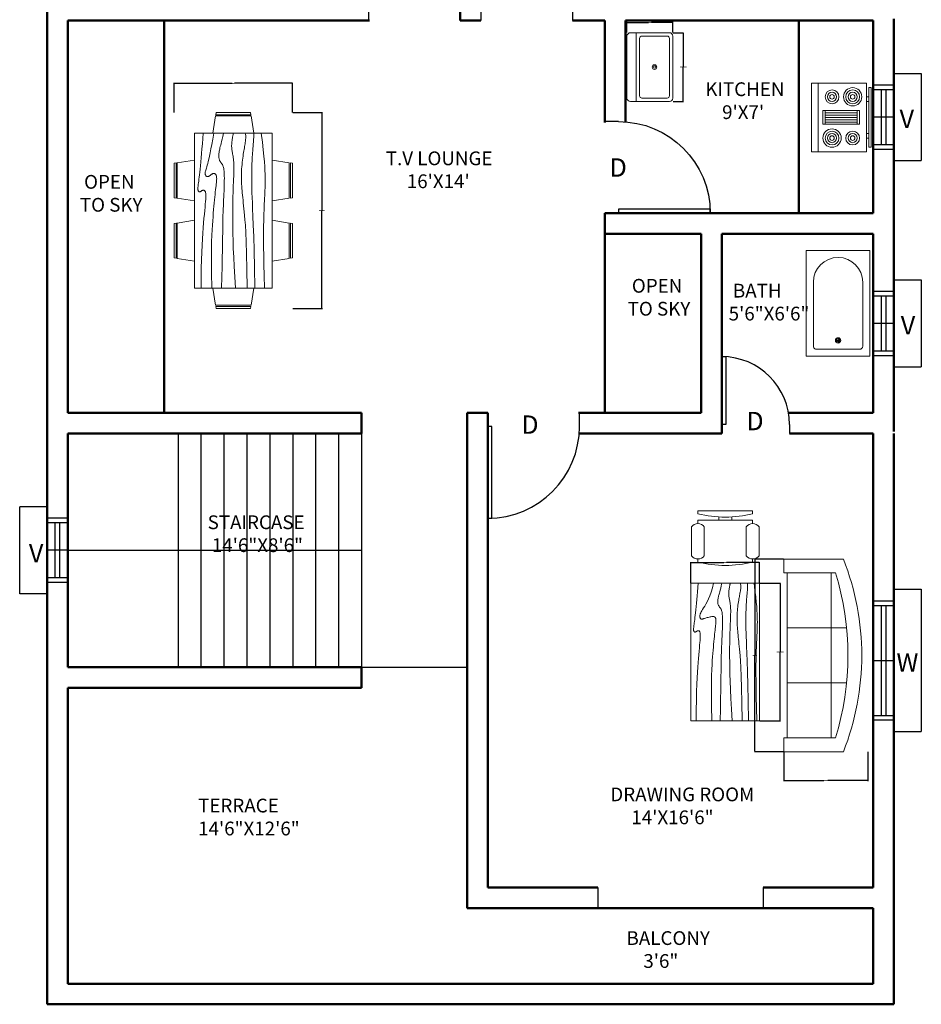
# Model space of a CAD drawing. Units: inches. Extents: x -8 to 1354, y -679 to 94.
# Tile 5 of 6: x 961 to 1354, y -679 to -249. Entities that reach past the tile are written whole.
import ezdxf

# ---------------------------------------------------------------- set-up
doc = ezdxf.new("R2010")
doc.units = ezdxf.units.IN
doc.header["$MEASUREMENT"] = 0
for name, color, linetype, lineweight in [('A-ANNO-DIMS', 2, 'Continuous', 18), ('A-ANNO-TEXT', 7, 'Continuous', 25), ('A-AREA-IDEN', 7, 'Continuous', 25), ('A-DOOR', 3, 'Continuous', 25), ('A-FLOR-FIXT', 8, 'Continuous', 18), ('A-FLOR-STRS', 2, 'Continuous', 25), ('A-FURN', 8, 'Continuous', 18), ('A-GLAZ', 4, 'Continuous', 25), ('A-WALL', 1, 'Continuous', 50)]:
    doc.layers.add(name, color=color, linetype=linetype, lineweight=lineweight)
doc.styles.get("Standard").update_dxf_attribs({"font": 'arial.ttf'})
doc.dimstyles.get("Standard").update_dxf_attribs({"dimtxt": 0.18, "dimasz": 0.18, "dimexe": 0.18, "dimexo": 0.0625, "dimgap": 0.09, "dimtad": 0, "dimtih": 1, "dimtoh": 1, "dimdec": 1, "dimzin": 0, "dimdsep": 46, "dimlunit": 4, "dimtxsty": 'Standard', "dimcen": 0.09, "dimclrd": 2, "dimclre": 3, "dimclrt": 6, "dimadec": 0, "dimazin": 0, "dimtfac": 1, "dimtdec": 1, "dimtofl": 0, "dimtmove": 0, "dimatfit": 3, "dimfxl": 1, "dimtfill": 2, "dimtfillclr": 4, "dimtolj": 1, "dimtzin": 0, "dimarcsym": 0})

# ---------------------------------------------------------------- blocks, each defined once
blk = doc.blocks.new('*U2')
for p, q in [((0, 0), (0, 6)), ((40, 0), (40, 6))]:
    blk.add_line(p, q)
blk.add_lwpolyline([(0, 0), (0, -40), (1.75, -40), (1.75, 0)], close=True)
blk.add_arc((0, 0), 40, 270, 0)
blk = doc.blocks.new('*U4')
for p, q in [((0, 0), (0, -100)), ((750, 0), (750, -100))]:
    blk.add_line(p, q)
blk.add_lwpolyline([(0, 0), (0, 750), (43.75, 750), (43.75, 0)], close=True)
blk.add_arc((0, 0), 750, 0, 90)
blk = doc.blocks.new('*U30')
for p, q in [((0, 0), (0, -6)), ((40, 0), (40, -6))]:
    blk.add_line(p, q)
blk.add_lwpolyline([(0, 0), (0, 40), (1.75, 40), (1.75, 0)], close=True)
blk.add_arc((0, 0), 40, 0, 90)
blk = doc.blocks.new('Sofa - Roundback 7 ft.')
for p, q in [((-12.00002, -32.4421), (-12.00003, -6.5971)), ((11.99997, -32.4421), (11.99998, -6.5971)), ((-36.000027, -34), (-36.000027, -11.4696)), ((35.99998, -34), (35.99998, -11.4696)), ((-35.999844, -13.3819), (35.9998, -13.3819)), ((-36.000027, -32.4421), (35.99998, -32.4421))]:
    blk.add_line(p, q)
for points in [[(-36.000027, -34), (-42.000027, -34), (-42.000027, -8)], [(41.99998, -8), (41.99998, -34), (35.99998, -34)]]:
    blk.add_lwpolyline(points)
for centre, radius, start, end in [((0, -114.25), 114.25, 68.43141, 111.5686), ((-0.00001, -127.1968), 121.1968, 72.72033, 107.2797)]:
    blk.add_arc(centre, radius, start, end)
blk = doc.blocks.new('Table - Rectangular Woodgrain 60 x 30 in.')
for p, q in [((0, 0), (0, -30)), ((60, 0), (0, 0)), ((60, -30), (60, 0)), ((0, -30), (60, -30))]:
    blk.add_line(p, q)
for points in [[(0, -2.4), (4.8155, -2.418), (9.0302, -2.4688), (12.709, -2.5477), (15.9167, -2.65), (18.7181, -2.7711), (21.1781, -2.9063), (23.3616, -3.0508), (25.3333, -3.2), (27.1477, -3.3495), (28.8172, -3.4958), (30.3437, -3.636), (31.7291, -3.7667), (32.9756, -3.8849), (34.0849, -3.9875), (35.059, -4.0714), (35.9, -4.1334), (36.6114, -4.1711), (37.2041, -4.1854), (37.6906, -4.1779), (38.0833, -4.15), (38.3948, -4.1034), (38.6375, -4.0396), (38.8239, -3.9602), (38.9666, -3.8667), (39.0764, -3.7608), (39.1573, -3.6448), (39.2116, -3.521), (39.2416, -3.3917), (39.2498, -3.2593), (39.2385, -3.1261), (39.21, -2.9944), (39.1666, -2.8667), (39.111, -2.7447), (39.0468, -2.6281), (38.978, -2.5163), (38.9083, -2.4083), (38.8418, -2.3035), (38.7823, -2.201), (38.7337, -2.1001), (38.7, -2), (38.6844, -1.9003), (38.6875, -1.8021), (38.7094, -1.707), (38.75, -1.6167), (38.8094, -1.5326), (38.8875, -1.4563), (38.9844, -1.3893), (39.1, -1.3333), (39.2351, -1.2896), (39.3937, -1.2583), (39.5804, -1.2396), (39.8, -1.2333), (40.057, -1.2396), (40.3562, -1.2583), (40.7023, -1.2896), (41.1, -1.3333), (41.5547, -1.3895), (42.0755, -1.4573), (42.6721, -1.5361), (43.3542, -1.625), (44.1316, -1.7233), (45.014, -1.8302), (46.0114, -1.9449), (47.1333, -2.0667), (48.3862, -2.1947), (49.7625, -2.3281), (51.2513, -2.4663), (52.8416, -2.6083), (54.5226, -2.7535), (56.2833, -2.9011), (58.1127, -3.0501), (60, -3.2)], [(0, -9.2), (6.5759, -9.0858), (11.9385, -9.0365), (16.2527, -9.0418), (19.6833, -9.0917), (22.3952, -9.1759), (24.5531, -9.2844), (26.322, -9.4069), (27.8666, -9.5333), (29.3241, -9.6553), (30.7203, -9.7719), (32.0532, -9.8837), (33.3208, -9.9917), (34.5213, -10.0965), (35.6526, -10.199), (36.7128, -10.2999), (37.7, -10.4), (38.6129, -10.4996), (39.4531, -10.5969), (40.223, -10.6895), (40.925, -10.775), (41.5613, -10.8512), (42.1344, -10.9156), (42.6465, -10.966), (43.1, -11), (43.4976, -11.0158), (43.8437, -11.0136), (44.143, -10.9942), (44.4, -10.9583), (44.6195, -10.9069), (44.8062, -10.8406), (44.9648, -10.7603), (45.1, -10.6667), (45.2155, -10.5598), (45.3114, -10.4365), (45.3871, -10.2929), (45.4416, -10.125), (45.4743, -9.929), (45.4844, -9.7011), (45.4709, -9.4371), (45.4333, -9.1333), (45.3716, -8.7883), (45.2896, -8.4104), (45.1919, -8.0107), (45.0833, -7.6), (44.9685, -7.1893), (44.8521, -6.7896), (44.7388, -6.4117), (44.6333, -6.0667), (44.54, -5.7628), (44.4614, -5.4979), (44.4001, -5.2675), (44.3583, -5.0667), (44.3384, -4.8909), (44.3427, -4.7354), (44.3736, -4.5956), (44.4333, -4.4667), (44.5236, -4.3453), (44.6427, -4.2333), (44.7884, -4.1339), (44.9583, -4.05), (45.1501, -3.9849), (45.3614, -3.9417), (45.59, -3.9234), (45.8333, -3.9333), (46.0915, -3.9749), (46.3734, -4.0531), (46.6906, -4.1736), (47.0542, -4.3417), (47.4756, -4.5629), (47.9661, -4.8427), (48.5372, -5.1866), (49.2, -5.6), (49.9676, -6.0844), (50.8594, -6.625), (51.8965, -7.2031), (53.1, -7.8), (54.491, -8.3969), (56.0906, -8.975), (57.9199, -9.5156), (60, -10)], [(0, -12.8), (5.1847, -12.9322), (9.6213, -13.0323), (13.3963, -13.1059), (16.5958, -13.1583), (19.3063, -13.1952), (21.614, -13.2219), (23.6054, -13.2439), (25.3666, -13.2667), (26.9728, -13.2947), (28.4531, -13.3281), (29.8256, -13.3663), (31.1083, -13.4083), (32.3191, -13.4535), (33.476, -13.501), (34.597, -13.5501), (35.7, -13.6), (36.7984, -13.6497), (37.8875, -13.6979), (38.9578, -13.743), (40, -13.7833), (41.0047, -13.8174), (41.9625, -13.8438), (42.864, -13.8607), (43.7, -13.8667), (44.4631, -13.8604), (45.1552, -13.8417), (45.7801, -13.8104), (46.3416, -13.7667), (46.8439, -13.7104), (47.2906, -13.6417), (47.6858, -13.5604), (48.0333, -13.4667), (48.3375, -13.3608), (48.6042, -13.2448), (48.8396, -13.121), (49.05, -12.9917), (49.2417, -12.8593), (49.4208, -12.7261), (49.5937, -12.5944), (49.7667, -12.4667), (49.9452, -12.3451), (50.1323, -12.2313), (50.3303, -12.1268), (50.5416, -12.0333), (50.7686, -11.9524), (51.0135, -11.8854), (51.2788, -11.8341), (51.5666, -11.8), (51.8785, -11.7843), (52.2116, -11.7865), (52.562, -11.8059), (52.926, -11.8417), (53.2998, -11.8931), (53.6795, -11.9594), (54.0614, -12.0397), (54.4416, -12.1333), (54.8223, -12.2401), (55.2293, -12.3625), (55.6942, -12.5037), (56.2489, -12.6667), (56.9251, -12.8547), (57.7545, -13.0708), (58.7689, -13.3182), (60, -13.6)], [(0, -18), (5.124, -17.7273), (9.6609, -17.5057), (13.6705, -17.3303), (17.2125, -17.1958), (20.3467, -17.0973), (23.1328, -17.0297), (25.6307, -16.9878), (27.9, -16.9667), (29.9928, -16.9617), (31.9302, -16.9703), (33.7254, -16.9907), (35.3917, -17.0208), (36.9423, -17.0588), (38.3906, -17.1026), (39.7499, -17.1503), (41.0333, -17.2), (42.2519, -17.2496), (43.4073, -17.2969), (44.4986, -17.3395), (45.525, -17.375), (46.4858, -17.4012), (47.3802, -17.4156), (48.2074, -17.416), (48.9667, -17.4), (49.6583, -17.3662), (50.2872, -17.3167), (50.8595, -17.2547), (51.3812, -17.1833), (51.8584, -17.1057), (52.2971, -17.025), (52.7034, -16.9443), (53.0833, -16.8667), (53.443, -16.7951), (53.789, -16.7313), (54.128, -16.6768), (54.4666, -16.6334), (54.8115, -16.6024), (55.1693, -16.5854), (55.5465, -16.5841), (55.95, -16.6), (56.3828, -16.6337), (56.8346, -16.6823), (57.2915, -16.7418), (57.7396, -16.8084), (58.165, -16.878), (58.5539, -16.9469), (58.8924, -17.0111), (59.1666, -17.0667), (59.3679, -17.1107), (59.5078, -17.1438), (59.6032, -17.1675), (59.6708, -17.1833), (59.7275, -17.193), (59.7901, -17.1979), (59.8753, -17.1998), (60, -17.2)], [(0, -22.4), (8.0098, -22.2501), (14.4094, -22.1011), (19.4168, -21.9535), (23.25, -21.8083), (26.1269, -21.6663), (28.2656, -21.5281), (29.884, -21.3947), (31.2, -21.2667), (32.3967, -21.1448), (33.5172, -21.0292), (34.5697, -20.9198), (35.5625, -20.8167), (36.5037, -20.7198), (37.4015, -20.6292), (38.2642, -20.5448), (39.1, -20.4667), (39.9164, -20.3951), (40.7187, -20.3313), (41.5117, -20.2768), (42.3, -20.2333), (43.0883, -20.2024), (43.8812, -20.1854), (44.6836, -20.1841), (45.5, -20.2), (46.3328, -20.234), (47.1747, -20.2844), (48.0163, -20.3488), (48.8479, -20.425), (49.66, -20.5106), (50.4429, -20.6031), (51.1872, -20.7004), (51.8833, -20.8), (52.5246, -20.8999), (53.1166, -20.9995), (53.6681, -21.0983), (54.1875, -21.1958), (54.6834, -21.2919), (55.1646, -21.3859), (55.6394, -21.4777), (56.1167, -21.5667), (56.6028, -21.6515), (57.0961, -21.7266), (57.5929, -21.7852), (58.0896, -21.8208), (58.5823, -21.8268), (59.0674, -21.7964), (59.5412, -21.723), (60, -21.6)], [(0, -25.2), (8.6355, -25.0504), (15.7026, -24.9031), (21.4049, -24.7606), (25.9458, -24.625), (29.529, -24.4988), (32.3578, -24.3844), (34.6359, -24.284), (36.5667, -24.2), (38.3213, -24.1341), (39.9417, -24.0854), (41.437, -24.0523), (42.8167, -24.0333), (44.0901, -24.0268), (45.2667, -24.0313), (46.3557, -24.0451), (47.3667, -24.0667), (48.309, -24.0947), (49.1928, -24.1287), (50.0284, -24.168), (50.826, -24.2125), (51.5959, -24.2617), (52.3483, -24.3151), (53.0935, -24.3725), (53.8417, -24.4334), (54.6009, -24.497), (55.3699, -24.561), (56.1454, -24.6226), (56.9239, -24.6792), (57.7021, -24.7279), (58.4764, -24.7662), (59.2435, -24.7911), (60, -24.8)], [(0, -28.8), (5.6867, -28.6681), (10.45, -28.5698), (14.407, -28.5012), (17.675, -28.4584), (20.3711, -28.4374), (22.6125, -28.4344), (24.5164, -28.4455), (26.2, -28.4667), (27.762, -28.4947), (29.2276, -28.5281), (30.6033, -28.5663), (31.8958, -28.6084), (33.1118, -28.6535), (34.2578, -28.7011), (35.3405, -28.7501), (36.3666, -28.8), (37.3443, -28.8497), (38.288, -28.8974), (39.2137, -28.9412), (40.1375, -28.9792), (41.0753, -29.0093), (42.0432, -29.0297), (43.0572, -29.0384), (44.1333, -29.0333), (45.2936, -29.0114), (46.5843, -28.9641), (48.0579, -28.8816), (49.7666, -28.7542), (51.7629, -28.5721), (54.0989, -28.3255), (56.8272, -28.0048), (60, -27.6)]]:
    blk.add_lwpolyline(points)
blk = doc.blocks.new('Chair - Desk')
for p, q in [((-8.5, 0), (-8.5, -1)), ((-8.5, 0), (8.5, 0)), ((8.5, 0), (8.5, -1)), ((-8.5, -3), (-8.5, -4)), ((-8.5, -3), (8.5, -3)), ((-2, -3), (-2, -1.9355)), ((2, -1.9576), (2, -3)), ((8.5, -3), (8.5, -4)), ((-10.5, -5), (-10.5, -14)), ((-6.5, -14), (-6.5, -5)), ((6.5, -5), (6.5, -14)), ((10.5, -14), (10.5, -5)), ((-8.5, -15), (-8.5, -16)), ((8.5, -15), (8.5, -16))]:
    blk.add_line(p, q)
for centre, radius, start, end in [((0, 34.625), 36.625, 256.5803, 283.4197), ((-8.5, -6.5), 2.5, 36.8699, 143.1301), ((8.5, -6.5), 2.5, 36.8699, 143.1301), ((-8.5, -12.5), 2.5, 216.8699, 323.1301), ((8.5, -12.5), 2.5, 216.8699, 323.1301), ((0, 19.625), 36.625, 256.5803, 283.4197)]:
    blk.add_arc(centre, radius, start, end)
blk = doc.blocks.new('Bath Tub - 26 x 60 in.')
for p, q in [((8, -18), (10, -18)), ((9, -17), (9, -19))]:
    blk.add_line(p, q)
blk.add_lwpolyline([(0, -36), (0, 0), (60, 0), (60, -36)], close=True)
for points in [[(6, -4), (42, -4)], [(4, -30), (4, -6)], [(42, -32), (6, -32)]]:
    blk.add_lwpolyline(points)
for radius in [1.5, 1]:
    blk.add_circle((9, -18), radius)
for centre, radius, start, end in [((5.75, -5.75), 1.77, 81.8699, 188.1301), ((42, -18), 14, 270, 90), ((5.75, -30.25), 1.77, 171.8699, 278.1301)]:
    blk.add_arc(centre, radius, start, end)
blk = doc.blocks.new('Range-Oven - 30 in top')
for p, q in [((0, -3), (30, -3)), ((12, -6), (18, -6)), ((13, -20), (13, -6)), ((14, -6), (14, -20)), ((15, -20), (15, -6)), ((16, -6), (16, -20)), ((17, -20), (17, -6)), ((18, -20), (12, -20)), ((6, -24), (6, -25)), ((8, -25), (8, -24)), ((22, -25), (22, -24)), ((24, -24), (24, -25))]:
    blk.add_line(p, q)
for points in [[(0, -24), (0, 0), (30, 0), (30, -24)], [(12, -21), (12, -5), (18, -5), (18, -21)], [(2, -26), (2, -25), (28, -25), (28, -26)]]:
    blk.add_lwpolyline(points, close=True)
for centre, radius in [((6, -9), 4), ((6, -9), 3), ((6, -9), 2), ((6, -9), 1), ((24, -9), 3), ((24, -9), 2), ((24, -9), 1), ((6, -18), 3), ((6, -18), 2), ((6, -18), 1), ((24, -18), 4), ((24, -18), 3), ((24, -18), 2), ((24, -18), 1)]:
    blk.add_circle(centre, radius)
blk = doc.blocks.new('Sink-single - 30 in top')
blk.add_line((-15, -3.999996), (15, -3.999996))
for points in [[(-13.5, 0), (13.5, 0)], [(-15, -18.499996), (-15, -1.5)], [(15, -1.5), (15, -18.499996)], [(-13.5, -17.499996), (-13.5, -6.499996)], [(-12.5, -5.499996), (12.5, -5.499996)], [(13.5, -6.499996), (13.5, -17.499996)], [(13.5, -19.999996), (-13.5, -19.999996)], [(12.5, -18.499996), (-12.5, -18.499996)]]:
    blk.add_lwpolyline(points)
for radius in [1, 0.5]:
    blk.add_circle((0, -11.999996), radius)
for centre, radius, start, end in [((-13.5, -1.5), 1.5, 90, 180), ((13.5, -1.5), 1.5, 0, 90), ((-12.5, -6.499996), 1, 90, 180), ((12.5, -6.499996), 1, 0, 90), ((-13.5, -18.499996), 1.5, 180, 270), ((-12.5, -17.499996), 1, 180, 270), ((12.5, -17.499996), 1, 270, 0), ((13.5, -18.499996), 1.5, 270, 0)]:
    blk.add_arc(centre, radius, start, end)
blk = doc.blocks.new('Dining Set - 36 x 72 in.')
for p, q in [((-22, 27.5), (-22.1562, 26.50042)), ((-22, 27.5), (-6, 27.5)), ((-5.8437, 26.49966), (-6, 27.5)), ((6, 27.5), (5.8438, 26.50042)), ((6, 27.5), (22, 27.5)), ((22.1563, 26.49966), (22, 27.5)), ((-22.2343, 26.00059), (-23.4847, 17.99762)), ((-22.2304, 26), (-5.7608, 26)), ((-5.8416, 26.5), (-22.1534, 26.5)), ((-4.5152, 17.99762), (-5.7655, 25.99926)), ((5.7657, 26.00059), (4.5153, 17.99762)), ((5.7696, 26), (22.2392, 26)), ((22.1584, 26.5), (5.8466, 26.5)), ((23.4848, 17.99762), (22.2345, 25.99926)), ((36, 18), (-36, 18)), ((-36, 18), (-36, -18)), ((36, -18), (36, 18)), ((-44.0006, 8.23428), (-35.9976, 9.48474)), ((44.0006, 8.23428), (35.9976, 9.48474)), ((-45.5, 8), (-44.5004, 8.15617)), ((-45.5, 8), (-45.5, -8)), ((-44.5, -8.15843), (-44.5, 8.15338)), ((-44, 8.23041), (-44, -8.23915)), ((44, 8.23041), (44, -8.23915)), ((44.5, -8.15843), (44.5, 8.15338)), ((45.5, 8), (44.5005, 8.15617)), ((45.5, 8), (45.5, -8)), ((-44.4997, -8.15631), (-45.5, -8)), ((-35.9976, -9.48476), (-43.9993, -8.2345)), ((35.9976, -9.48476), (43.9993, -8.2345)), ((44.4997, -8.15631), (45.5, -8)), ((-36, -18), (36, -18)), ((-22.2343, -26.0006), (-23.4847, -17.99762)), ((-4.5152, -17.99762), (-5.7655, -25.99928)), ((5.7657, -26.0006), (4.5153, -17.99762)), ((23.4848, -17.99762), (22.2345, -25.99928)), ((-22.2304, -26), (-5.7608, -26)), ((-22, -27.5), (-22.1562, -26.50044)), ((-5.8416, -26.5), (-22.1534, -26.5)), ((-5.8437, -26.49967), (-6, -27.5)), ((5.7696, -26), (22.2392, -26)), ((6, -27.5), (5.8438, -26.50044)), ((22.1584, -26.5), (5.8466, -26.5)), ((22.1563, -26.49967), (22, -27.5)), ((-22, -27.5), (-6, -27.5)), ((6, -27.5), (22, -27.5))]:
    blk.add_line(p, q)
for points in [[(-36, 15), (-31.1772, 14.97754), (-26.8079, 14.91406), (-22.8538, 14.81543), (-19.276, 14.6875), (-16.0362, 14.53613), (-13.0957, 14.36718), (-10.4159, 14.18652), (-7.9583, 14), (-5.6904, 13.81315), (-3.6035, 13.63021), (-1.6954, 13.45508), (0.0365, 13.29166), (1.5945, 13.14388), (2.9811, 13.01562), (4.1988, 12.9108), (5.25, 12.83333), (6.1393, 12.78613), (6.8802, 12.76823), (7.4883, 12.77767), (7.9792, 12.8125), (8.3685, 12.87077), (8.6719, 12.95052), (8.9049, 13.0498), (9.0833, 13.16666), (9.2205, 13.29899), (9.3216, 13.44401), (9.3895, 13.59879), (9.4271, 13.76041), (9.4373, 13.92594), (9.4232, 14.09245), (9.3875, 14.257), (9.3333, 14.41666), (9.2638, 14.56917), (9.1836, 14.71484), (9.0975, 14.85465), (9.0104, 14.98958), (8.9272, 15.1206), (8.8529, 15.2487), (8.7922, 15.37483), (8.75, 15.5), (8.7305, 15.62467), (8.7344, 15.74739), (8.7617, 15.86621), (8.8125, 15.97916), (8.8867, 16.08431), (8.9844, 16.17968), (9.1055, 16.26334), (9.25, 16.33333), (9.4189, 16.38802), (9.6172, 16.42708), (9.8506, 16.45052), (10.125, 16.45833), (10.4463, 16.45052), (10.8203, 16.42708), (11.2529, 16.38802), (11.75, 16.33333), (12.3184, 16.26318), (12.9694, 16.17838), (13.7151, 16.07991), (14.5677, 15.96875), (15.5395, 15.84586), (16.6426, 15.71224), (17.8893, 15.56884), (19.2917, 15.41666), (20.859, 15.25667), (22.5879, 15.08984), (24.4721, 14.91715), (26.5052, 14.73958), (28.6809, 14.5581), (30.9929, 14.3737), (33.4347, 14.18733), (36, 14)], [(-36, 10), (-28.9766, 10.14274), (-23.1725, 10.20442), (-18.4241, 10.19775), (-14.5677, 10.13541), (-11.4399, 10.03011), (-8.877, 9.89453), (-6.7154, 9.74137), (-4.7917, 9.58333), (-2.9698, 9.43082), (-1.2246, 9.28515), (0.4415, 9.14534), (2.026, 9.01041), (3.5266, 8.87939), (4.9408, 8.7513), (6.266, 8.62516), (7.5, 8.5), (8.6411, 8.37549), (9.6914, 8.2539), (10.6538, 8.13818), (11.5312, 8.03125), (12.3267, 7.93603), (13.043, 7.85547), (13.6831, 7.79248), (14.25, 7.75), (14.7471, 7.7303), (15.1797, 7.73307), (15.5537, 7.75732), (15.875, 7.80208), (16.1494, 7.86637), (16.3828, 7.94922), (16.5811, 8.04964), (16.75, 8.16666), (16.8944, 8.29915), (17.0143, 8.44531), (17.1089, 8.60319), (17.1771, 8.77083), (17.218, 8.94629), (17.2305, 9.1276), (17.2137, 9.31282), (17.1667, 9.5), (17.0895, 9.6875), (16.987, 9.875), (16.8649, 10.0625), (16.7292, 10.25), (16.5856, 10.4375), (16.4401, 10.625), (16.2985, 10.8125), (16.1667, 11), (16.05, 11.18733), (15.9518, 11.3737), (15.8752, 11.5581), (15.8229, 11.73958), (15.798, 11.91715), (15.8034, 12.08984), (15.842, 12.25667), (15.9167, 12.41666), (16.0295, 12.56836), (16.1784, 12.70833), (16.3605, 12.83268), (16.5729, 12.9375), (16.8127, 13.01888), (17.0768, 13.07291), (17.3625, 13.0957), (17.6667, 13.08333), (17.9894, 13.03312), (18.3418, 12.94726), (18.7382, 12.82918), (19.1927, 12.68229), (19.7195, 12.51001), (20.3327, 12.31575), (21.0465, 12.10294), (21.875, 11.875), (22.8357, 11.63354), (23.959, 11.37304), (25.2786, 11.08618), (26.8282, 10.76562), (28.6414, 10.40405), (30.752, 9.99414), (33.1936, 9.52856), (36, 9)], [(-36, 5.5), (-30.7157, 5.3348), (-26.069, 5.20963), (-21.9946, 5.11767), (-18.4271, 5.05208), (-15.3009, 5.00602), (-12.5508, 4.97265), (-10.1112, 4.94515), (-7.9167, 4.91666), (-5.909, 4.88167), (-4.0586, 4.83984), (-2.3429, 4.79215), (-0.7396, 4.73958), (0.7739, 4.6831), (2.22, 4.6237), (3.6213, 4.56233), (5, 4.5), (6.373, 4.43782), (7.7344, 4.3776), (9.0723, 4.32129), (10.375, 4.27083), (11.6309, 4.22819), (12.8281, 4.19531), (13.9551, 4.17415), (15, 4.16666), (15.954, 4.17448), (16.819, 4.19791), (17.6001, 4.23698), (18.3021, 4.29166), (18.9299, 4.36198), (19.4883, 4.44791), (19.9823, 4.54948), (20.4167, 4.66666), (20.7969, 4.79899), (21.1302, 4.94401), (21.4245, 5.09879), (21.6875, 5.26041), (21.9271, 5.42594), (22.1511, 5.59245), (22.3672, 5.757), (22.5834, 5.91666), (22.8065, 6.06868), (23.0404, 6.21093), (23.2879, 6.34147), (23.5521, 6.45833), (23.8358, 6.55957), (24.142, 6.64323), (24.4735, 6.70735), (24.8334, 6.75), (25.2235, 6.76969), (25.642, 6.76692), (26.0858, 6.74267), (26.5521, 6.69791), (27.0379, 6.63362), (27.5404, 6.55078), (28.0565, 6.45036), (28.5834, 6.33333), (29.1242, 6.19987), (29.7071, 6.04687), (30.3661, 5.87044), (31.1354, 5.66666), (32.0493, 5.43164), (33.142, 5.16146), (34.4475, 4.85221), (36, 4.5)], [(-36, -1), (-30.7915, -0.6591), (-26.0195, -0.38216), (-21.6519, -0.16284), (-17.6563, 0.00521), (-14.0005, 0.12833), (-10.6523, 0.21289), (-7.5796, 0.26522), (-4.75, 0.29166), (-2.134, 0.29793), (0.2878, 0.28711), (2.5317, 0.26163), (4.6146, 0.22396), (6.5529, 0.17651), (8.3633, 0.12174), (10.0623, 0.06209), (11.6667, 0), (13.1899, -0.06201), (14.6341, -0.1211), (15.9982, -0.17432), (17.2813, -0.21875), (18.4823, -0.25147), (19.6003, -0.26953), (20.6343, -0.27002), (21.5834, -0.25), (22.4481, -0.20768), (23.2357, -0.14584), (23.9549, -0.06836), (24.6146, 0.02083), (25.2235, 0.11784), (25.7904, 0.21875), (26.3241, 0.31966), (26.8334, 0.41666), (27.3265, 0.50618), (27.8099, 0.58593), (28.2894, 0.65397), (28.7709, 0.70833), (29.2601, 0.74707), (29.763, 0.76823), (30.2855, 0.76985), (30.8334, 0.75), (31.4088, 0.70784), (31.9994, 0.64713), (32.589, 0.57275), (33.1615, 0.48958), (33.7008, 0.4025), (34.1908, 0.3164), (34.6153, 0.23616), (34.9584, 0.16666), (35.2099, 0.11165), (35.3848, 0.07031), (35.504, 0.04069), (35.5886, 0.02083), (35.6594, 0.00879), (35.7377, 0.0026), (35.8442, 0.00032), (36, 0)], [(-36, -6.5), (-27.1843, -6.31267), (-20.084, -6.1263), (-14.469, -5.9419), (-10.1094, -5.76042), (-6.7752, -5.58285), (-4.2363, -5.41016), (-2.2629, -5.24333), (-0.625, -5.08334), (0.8708, -4.93099), (2.2715, -4.78646), (3.5872, -4.64974), (4.8281, -4.52084), (6.0046, -4.39974), (7.127, -4.28646), (8.2053, -4.18099), (9.25, -4.08334), (10.2705, -3.99382), (11.2734, -3.91407), (12.2647, -3.84603), (13.25, -3.79167), (14.2354, -3.75293), (15.2266, -3.73177), (16.2295, -3.73015), (17.25, -3.75), (18.2912, -3.79248), (19.3451, -3.85547), (20.4009, -3.93604), (21.4479, -4.03125), (22.4754, -4.13819), (23.4727, -4.25391), (24.4289, -4.37549), (25.3334, -4.5), (26.1785, -4.62492), (26.9694, -4.74935), (27.7145, -4.87281), (28.4219, -4.99479), (29.1, -5.11483), (29.7572, -5.23242), (30.4016, -5.34709), (31.0417, -5.45834), (31.6837, -5.56437), (32.3262, -5.65821), (32.9658, -5.73153), (33.599, -5.77604), (34.2224, -5.78345), (34.8327, -5.74545), (35.4264, -5.65373), (36, -5.5)], [(-36, -10), (-26.4022, -9.81299), (-18.4675, -9.62891), (-11.9839, -9.45069), (-6.7396, -9.28125), (-2.5226, -9.12354), (0.8789, -8.98047), (3.6769, -8.85498), (6.0833, -8.75), (8.2767, -8.66765), (10.3021, -8.60677), (12.1712, -8.56543), (13.8958, -8.54167), (15.4876, -8.53353), (16.9583, -8.53907), (18.3197, -8.55632), (19.5834, -8.58334), (20.7616, -8.61841), (21.8685, -8.66081), (22.9188, -8.71004), (23.9271, -8.76563), (24.9081, -8.82707), (25.8763, -8.89388), (26.8465, -8.96558), (27.8334, -9.04167), (28.8474, -9.12118), (29.8828, -9.20117), (30.93, -9.27824), (31.9792, -9.34896), (33.0205, -9.40991), (34.0443, -9.45768), (35.0407, -9.48885), (36, -9.5)], [(-36, -14.5), (-30.0881, -14.33513), (-25.0332, -14.21224), (-20.7312, -14.12647), (-17.0781, -14.07292), (-13.97, -14.04671), (-11.3027, -14.04297), (-8.9724, -14.05681), (-6.875, -14.08334), (-4.9224, -14.11833), (-3.0905, -14.16016), (-1.3709, -14.20785), (0.2448, -14.26042), (1.7647, -14.3169), (3.1973, -14.3763), (4.5507, -14.43767), (5.8333, -14.5), (7.0554, -14.5621), (8.235, -14.62175), (9.3922, -14.67652), (10.5469, -14.72396), (11.7192, -14.76164), (12.929, -14.78711), (14.1965, -14.79794), (15.5417, -14.79167), (16.9933, -14.76424), (18.6152, -14.70508), (20.4804, -14.60197), (22.6615, -14.44271), (25.2312, -14.21509), (28.2624, -13.9069), (31.8277, -13.50594), (36, -13)]]:
    blk.add_lwpolyline(points)
blk = doc.blocks.new('WIN-W')
at = {"ltscale": 2}
for p, q in [((12, 62), (0, 62)), ((0, 0), (0, 62)), ((12, 57), (12, 62)), ((12, 5), (12, 0)), ((12, 0), (0, 0))]:
    blk.add_line(p, q, dxfattribs=at)
for p, q in [((21, 57), (12, 57)), ((21, 5), (12, 5))]:
    blk.add_line(p, q)
blk = doc.blocks.new('VENT-V')
for p, q in [((0, 9), (0, 21)), ((0, 21), (38, 21)), ((38, 9), (38, 21)), ((5, 9), (0, 9)), ((5, 0), (5, 9)), ((33, 0), (33, 9)), ((33, 9), (38, 9))]:
    blk.add_line(p, q)
blk = doc.blocks.new('*D101')
at = {"layer": 'A-ANNO-DIMS', "color": 3, "lineweight": -2, "transparency": 16777216}
for p, q in [((1283.34, -494.98), (1292.45, -494.98)), ((1283.34, -554.98), (1292.45, -554.98))]:
    blk.add_line(p, q, dxfattribs=at)
at = {"layer": 'A-ANNO-DIMS', "color": 2, "lineweight": -2, "transparency": 16777216}
for p, q in [((1292.27, -495.16), (1292.27, -524.79)), ((1292.27, -554.8), (1292.27, -525.16))]:
    blk.add_line(p, q, dxfattribs=at)
at = {"layer": 'A-ANNO-DIMS', "color": 2, "transparency": 16777216}
for points in [[(1292.24, -495.16), (1292.3, -495.16), (1292.27, -494.98)], [(1292.24, -554.8), (1292.3, -554.8), (1292.27, -554.98)]]:
    blk.add_solid(points, dxfattribs=at)
at = {"layer": 'Defpoints', "color": 0, "transparency": 16777216}
for p in [(1283.27, -494.98), (1292.27, -494.98), (1283.27, -554.98)]:
    blk.add_point(p, dxfattribs=at)
at = {"layer": 'A-ANNO-DIMS', "color": 6, "transparency": 16777216, "insert": (1292.27, -524.98), "char_height": 0.18, "attachment_point": 5, "bg_fill": 1, "box_fill_scale": 1.25, "bg_fill_color": 4, "bg_fill_transparency": 0}
blk.add_mtext('\\A1;COFFEE TABLE 5\'-0" TYP.', dxfattribs=at)
blk = doc.blocks.new('*D102')
at = {"layer": 'A-ANNO-DIMS', "color": 3, "lineweight": -2, "transparency": 16777216}
for p, q in [((1253.27, -494.91), (1253.27, -485.8)), ((1283.27, -494.91), (1283.27, -485.8))]:
    blk.add_line(p, q, dxfattribs=at)
at = {"layer": 'A-ANNO-DIMS', "color": 2, "lineweight": -2, "transparency": 16777216}
for p, q in [((1253.45, -485.98), (1267.63, -485.98)), ((1283.09, -485.98), (1268.91, -485.98))]:
    blk.add_line(p, q, dxfattribs=at)
at = {"layer": 'A-ANNO-DIMS', "color": 2, "transparency": 16777216}
for points in [[(1253.45, -485.95), (1253.45, -486.01), (1253.27, -485.98)], [(1283.09, -485.95), (1283.09, -486.01), (1283.27, -485.98)]]:
    blk.add_solid(points, dxfattribs=at)
at = {"layer": 'Defpoints', "color": 0, "transparency": 16777216}
for p in [(1253.27, -485.98), (1253.27, -494.98), (1283.27, -494.98)]:
    blk.add_point(p, dxfattribs=at)
at = {"layer": 'A-ANNO-DIMS', "color": 6, "transparency": 16777216, "insert": (1268.27, -485.98), "char_height": 0.18, "attachment_point": 5, "bg_fill": 1, "box_fill_scale": 1.25, "bg_fill_color": 4, "bg_fill_transparency": 0}
blk.add_mtext('\\A1;2\'-6" TYP.', dxfattribs=at)
blk = doc.blocks.new('*D105')
at = {"layer": 'A-ANNO-DIMS', "color": 3, "lineweight": -2, "transparency": 16777216}
for p, q in [((1079.77, -289.78), (1092.7, -289.78)), ((1079.77, -375.2), (1092.7, -375.2))]:
    blk.add_line(p, q, dxfattribs=at)
at = {"layer": 'A-ANNO-DIMS', "color": 2, "lineweight": -2, "transparency": 16777216}
for p, q in [((1092.52, -289.96), (1092.52, -332.31)), ((1092.52, -375.02), (1092.52, -332.68))]:
    blk.add_line(p, q, dxfattribs=at)
at = {"layer": 'A-ANNO-DIMS', "color": 2, "transparency": 16777216}
for points in [[(1092.49, -289.96), (1092.55, -289.96), (1092.52, -289.78)], [(1092.49, -375.02), (1092.55, -375.02), (1092.52, -375.2)]]:
    blk.add_solid(points, dxfattribs=at)
at = {"layer": 'Defpoints', "color": 0, "transparency": 16777216}
for p in [(1079.7, -289.78), (1092.52, -289.78), (1079.7, -375.2)]:
    blk.add_point(p, dxfattribs=at)
at = {"layer": 'A-ANNO-DIMS', "color": 6, "transparency": 16777216, "insert": (1092.52, -332.49), "char_height": 0.18, "attachment_point": 5, "bg_fill": 1, "box_fill_scale": 1.25, "bg_fill_color": 4, "bg_fill_transparency": 0}
blk.add_mtext('\\A1;DINING SET 7\'-1 1/2"', dxfattribs=at)
blk = doc.blocks.new('*D106')
at = {"layer": 'A-ANNO-DIMS', "color": 3, "lineweight": -2, "transparency": 16777216}
for p, q in [((1028.08, -289.72), (1028.08, -276.79)), ((1079.7, -289.72), (1079.7, -276.79))]:
    blk.add_line(p, q, dxfattribs=at)
at = {"layer": 'A-ANNO-DIMS', "color": 2, "lineweight": -2, "transparency": 16777216}
for p, q in [((1028.26, -276.97), (1053.35, -276.97)), ((1079.52, -276.97), (1054.43, -276.97))]:
    blk.add_line(p, q, dxfattribs=at)
at = {"layer": 'A-ANNO-DIMS', "color": 2, "transparency": 16777216}
for points in [[(1028.26, -276.94), (1028.26, -277), (1028.08, -276.97)], [(1079.52, -276.94), (1079.52, -277), (1079.7, -276.97)]]:
    blk.add_solid(points, dxfattribs=at)
at = {"layer": 'Defpoints', "color": 0, "transparency": 16777216}
for p in [(1028.08, -276.97), (1028.08, -289.78), (1079.7, -289.78)]:
    blk.add_point(p, dxfattribs=at)
at = {"layer": 'A-ANNO-DIMS', "color": 6, "transparency": 16777216, "insert": (1053.89, -276.97), "char_height": 0.18, "attachment_point": 5, "bg_fill": 1, "box_fill_scale": 1.25, "bg_fill_color": 4, "bg_fill_transparency": 0}
blk.add_mtext('\\A1;4\'-3 1/2"', dxfattribs=at)
blk = doc.blocks.new('*D109')
at = {"layer": 'A-ANNO-DIMS', "color": 3, "lineweight": -2, "transparency": 16777216}
for p, q in [((1245.55, -254.9), (1250.17, -254.9)), ((1245.55, -284.9), (1250.17, -284.9))]:
    blk.add_line(p, q, dxfattribs=at)
at = {"layer": 'A-ANNO-DIMS', "color": 2, "lineweight": -2, "transparency": 16777216}
for p, q in [((1249.99, -255.08), (1249.99, -269.72)), ((1249.99, -284.72), (1249.99, -270.08))]:
    blk.add_line(p, q, dxfattribs=at)
at = {"layer": 'A-ANNO-DIMS', "color": 2, "transparency": 16777216}
for points in [[(1249.96, -255.08), (1250.02, -255.08), (1249.99, -254.9)], [(1249.96, -284.72), (1250.02, -284.72), (1249.99, -284.9)]]:
    blk.add_solid(points, dxfattribs=at)
at = {"layer": 'Defpoints', "color": 0, "transparency": 16777216}
for p in [(1245.49, -254.9), (1249.99, -254.9), (1245.49, -284.9)]:
    blk.add_point(p, dxfattribs=at)
at = {"layer": 'A-ANNO-DIMS', "color": 6, "transparency": 16777216, "insert": (1249.99, -269.9), "char_height": 0.18, "attachment_point": 5, "bg_fill": 1, "box_fill_scale": 1.25, "bg_fill_color": 4, "bg_fill_transparency": 0}
blk.add_mtext('\\A1;KITCHEN SINK 2\'-6" TYP.', dxfattribs=at)
blk = doc.blocks.new('*D110')
at = {"layer": 'A-ANNO-DIMS', "color": 3, "lineweight": -2, "transparency": 16777216}
for p, q in [((1225.49, -254.84), (1225.49, -250.22)), ((1245.49, -254.84), (1245.49, -250.22))]:
    blk.add_line(p, q, dxfattribs=at)
at = {"layer": 'A-ANNO-DIMS', "color": 2, "lineweight": -2, "transparency": 16777216}
for p, q in [((1225.67, -250.4), (1234.86, -250.4)), ((1245.31, -250.4), (1236.12, -250.4))]:
    blk.add_line(p, q, dxfattribs=at)
at = {"layer": 'A-ANNO-DIMS', "color": 2, "transparency": 16777216}
for points in [[(1225.67, -250.37), (1225.67, -250.43), (1225.49, -250.4)], [(1245.31, -250.37), (1245.31, -250.43), (1245.49, -250.4)]]:
    blk.add_solid(points, dxfattribs=at)
at = {"layer": 'Defpoints', "color": 0, "transparency": 16777216}
for p in [(1225.49, -250.4), (1225.49, -254.9), (1245.49, -254.9)]:
    blk.add_point(p, dxfattribs=at)
at = {"layer": 'A-ANNO-DIMS', "color": 6, "transparency": 16777216, "insert": (1235.49, -250.4), "char_height": 0.18, "attachment_point": 5, "bg_fill": 1, "box_fill_scale": 1.25, "bg_fill_color": 4, "bg_fill_transparency": 0}
blk.add_mtext('\\A1;1\'-8" TYP.', dxfattribs=at)
blk = doc.blocks.new('*D113')
at = {"layer": 'A-ANNO-DIMS', "color": 3, "lineweight": -2, "transparency": 16777216}
for p, q in [((1293.76, -484.48), (1281.04, -484.48)), ((1293.76, -568.48), (1281.04, -568.48))]:
    blk.add_line(p, q, dxfattribs=at)
at = {"layer": 'A-ANNO-DIMS', "color": 2, "lineweight": -2, "transparency": 16777216}
for p, q in [((1281.22, -484.66), (1281.22, -526.3)), ((1281.22, -568.3), (1281.22, -526.67))]:
    blk.add_line(p, q, dxfattribs=at)
at = {"layer": 'A-ANNO-DIMS', "color": 2, "transparency": 16777216}
for points in [[(1281.19, -484.66), (1281.25, -484.66), (1281.22, -484.48)], [(1281.19, -568.3), (1281.25, -568.3), (1281.22, -568.48)]]:
    blk.add_solid(points, dxfattribs=at)
at = {"layer": 'Defpoints', "color": 0, "transparency": 16777216}
for p in [(1293.82, -484.48), (1281.22, -568.48), (1293.82, -568.48)]:
    blk.add_point(p, dxfattribs=at)
at = {"layer": 'A-ANNO-DIMS', "color": 6, "transparency": 16777216, "insert": (1281.22, -526.48), "char_height": 0.18, "attachment_point": 5, "bg_fill": 1, "box_fill_scale": 1.25, "bg_fill_color": 4, "bg_fill_transparency": 0}
blk.add_mtext('\\A1;SOFA 7\'-0" TYP.', dxfattribs=at)
blk = doc.blocks.new('*D114')
at = {"layer": 'A-ANNO-DIMS', "color": 3, "lineweight": -2, "transparency": 16777216}
for p, q in [((1293.82, -568.55), (1293.82, -581.26)), ((1330.49, -568.55), (1330.49, -581.26))]:
    blk.add_line(p, q, dxfattribs=at)
at = {"layer": 'A-ANNO-DIMS', "color": 2, "lineweight": -2, "transparency": 16777216}
for p, q in [((1294, -581.08), (1311.3, -581.08)), ((1330.31, -581.08), (1313, -581.08))]:
    blk.add_line(p, q, dxfattribs=at)
at = {"layer": 'A-ANNO-DIMS', "color": 2, "transparency": 16777216}
for points in [[(1294, -581.05), (1294, -581.11), (1293.82, -581.08)], [(1330.31, -581.05), (1330.31, -581.11), (1330.49, -581.08)]]:
    blk.add_solid(points, dxfattribs=at)
at = {"layer": 'Defpoints', "color": 0, "transparency": 16777216}
for p in [(1293.82, -568.48), (1330.49, -568.48), (1330.49, -581.08)]:
    blk.add_point(p, dxfattribs=at)
at = {"layer": 'A-ANNO-DIMS', "color": 6, "transparency": 16777216, "insert": (1312.15, -581.08), "char_height": 0.18, "attachment_point": 5, "bg_fill": 1, "box_fill_scale": 1.25, "bg_fill_color": 4, "bg_fill_transparency": 0}
blk.add_mtext('\\A1;3\'-0 1/2" TYP.', dxfattribs=at)

msp = doc.modelspace()

# ---------------------------------------------------------------- linework, layer by layer
at = {"layer": 'A-FLOR-STRS'}
for p, q in [((1029.78, -429.65), (1029.78, -531.65)), ((1039.78, -429.65), (1039.78, -531.65)), ((1049.78, -429.65), (1049.78, -531.65)), ((1059.78, -429.65), (1059.78, -531.65)), ((1069.78, -429.65), (1069.78, -531.65)), ((1079.78, -429.65), (1079.78, -531.65)), ((1089.78, -429.65), (1089.78, -531.65)), ((1099.78, -429.65), (1099.78, -531.65)), ((1109.78, -429.65), (1109.78, -531.65)), ((981.78, -480.65), (1109.78, -480.65)), ((1109.78, -531.65), (1155.78, -531.65))]:
    msp.add_line(p, q, dxfattribs=at)
at = {"layer": 'A-GLAZ'}
for p, q in [((1332.78, -279.65), (1341.78, -279.65)), ((1336.28, -279.65), (1336.28, -303.65)), ((1338.28, -279.65), (1338.28, -303.65)), ((1332.78, -291.65), (1341.78, -291.65)), ((1332.78, -303.65), (1341.78, -303.65)), ((1332.78, -369.65), (1341.78, -369.65)), ((1336.28, -369.65), (1336.28, -393.65)), ((1338.28, -369.65), (1338.28, -393.65)), ((1332.78, -381.65), (1341.78, -381.65)), ((1332.78, -393.65), (1341.78, -393.65)), ((981.78, -468.65), (972.78, -468.65)), ((976.28, -492.65), (976.28, -468.65)), ((978.28, -492.65), (978.28, -468.65)), ((981.78, -480.65), (972.78, -480.65)), ((981.78, -492.65), (972.78, -492.65)), ((1332.78, -504.65), (1341.78, -504.65)), ((1336.28, -504.65), (1336.28, -552.65)), ((1338.28, -504.65), (1338.28, -552.65)), ((1332.78, -528.65), (1341.78, -528.65)), ((1332.78, -552.65), (1341.78, -552.65)), ((1212.78, -627.65), (1212.78, -636.65)), ((1284.78, -627.65), (1284.78, -636.65))]:
    msp.add_line(p, q, dxfattribs=at)
at = {"layer": 'A-WALL'}
for p, q in [((972.78, -60.65), (972.78, -429.65)), ((1152.78, -249.65), (1152.78, -60.65)), ((1341.78, -248.83), (1341.78, -333.65)), ((981.78, -249.65), (981.78, -420.65)), ((981.78, -249.65), (1023.78, -249.65)), ((1023.78, -249.65), (1113.23, -249.65)), ((1023.78, -420.65), (1023.78, -249.65)), ((1152.78, -249.65), (1161.78, -249.65)), ((1201.78, -249.65), (1215.78, -249.65)), ((1215.78, -294.1), (1215.78, -249.65)), ((1224.78, -249.65), (1332.78, -249.65)), ((1224.78, -293.76), (1224.78, -249.65)), ((1300.41, -249.65), (1300.41, -333.65)), ((1332.78, -249.65), (1332.78, -333.65)), ((1332.78, -333.65), (1215.78, -333.65)), ((1215.78, -420.65), (1215.78, -333.65)), ((1341.78, -333.65), (1341.78, -428.83)), ((1257.78, -342.65), (1215.78, -342.65)), ((1257.78, -420.65), (1257.78, -342.65)), ((1332.78, -342.65), (1266.78, -342.65)), ((1266.78, -429.65), (1266.78, -342.65)), ((1332.78, -342.65), (1332.78, -420.65)), ((1023.78, -420.65), (981.78, -420.65)), ((1109.78, -420.65), (1023.78, -420.65)), ((1109.78, -420.65), (1109.78, -429.65)), ((1164.78, -420.65), (1155.78, -420.65)), ((1155.78, -540.65), (1155.78, -420.65)), ((1164.78, -627.65), (1164.78, -420.65)), ((1215.78, -420.65), (1204.32, -420.65)), ((1257.78, -420.65), (1215.78, -420.65)), ((1266.95, -420.65), (1266.78, -420.65)), ((1332.78, -420.65), (1295.87, -420.65)), ((972.78, -429.65), (972.78, -678.65)), ((1109.78, -429.65), (981.78, -429.65)), ((1109.78, -429.65), (981.78, -429.65)), ((981.78, -429.65), (981.78, -531.65)), ((981.78, -429.65), (981.78, -531.65)), ((1215.78, -429.65), (1204.66, -429.65)), ((1266.78, -429.65), (1215.78, -429.65)), ((1332.78, -429.65), (1296.3, -429.65)), ((1332.78, -429.65), (1332.78, -627.65)), ((1341.78, -429.65), (1341.78, -636.65)), ((981.78, -531.65), (1109.78, -531.65)), ((1109.78, -540.65), (1109.78, -531.65)), ((981.78, -540.65), (981.78, -669.65)), ((981.78, -540.65), (1109.78, -540.65)), ((1155.78, -636.65), (1155.78, -540.65)), ((1212.78, -627.65), (1164.78, -627.65)), ((1332.78, -627.65), (1284.78, -627.65)), ((1212.78, -636.65), (1155.78, -636.65)), ((1212.78, -636.65), (1284.78, -636.65)), ((1332.78, -636.65), (1284.78, -636.65)), ((1332.78, -636.65), (1332.78, -669.65)), ((1341.78, -636.65), (1341.78, -678.65)), ((1332.78, -669.65), (981.78, -669.65)), ((1341.78, -678.65), (972.78, -678.65))]:
    msp.add_line(p, q, dxfattribs=at)

# ---------------------------------------------------------------- block references
at = {"layer": 'A-DOOR', "xscale": -1}
msp.add_blockref('*U30', (1152.78, -243.65), dxfattribs=at)
at = {"layer": 'A-DOOR'}
for name, p in [('*U30', (1161.78, -243.65)), ('*U2', (1164.78, -426.65))]:
    msp.add_blockref(name, p, dxfattribs=at)
at = {"layer": 'A-DOOR', "xscale": -1, "rotation": 270}
msp.add_blockref('*U30', (1221.78, -333.65), dxfattribs=at)
at = {"layer": 'A-DOOR', "xscale": 0.0393700787401575, "yscale": 0.0393700787401575, "zscale": 0.0393700787401575}
msp.add_blockref('*U4', (1266.78, -425.71), dxfattribs=at)
at = {"layer": 'A-FLOR-FIXT', "rotation": 90}
for name, p in [('Sink-single - 30 in top', (1225.49, -269.9)), ('Range-Oven - 30 in top', (1305.86, -306.87))]:
    msp.add_blockref(name, p, dxfattribs=at)
at = {"layer": 'A-FLOR-FIXT', "xscale": 0.76936780151118, "yscale": 0.76936780151118, "zscale": 0.76936780151118, "rotation": 90}
msp.add_blockref('Bath Tub - 26 x 60 in.', (1303.65, -396.02), dxfattribs=at)
at = {"layer": 'A-FURN', "xscale": 0.9386837105660525, "yscale": 0.9386837105660525, "zscale": 0.9386837105660525, "rotation": 90}
msp.add_blockref('Dining Set - 36 x 72 in.', (1053.89, -332.49), dxfattribs=at)
at = {"layer": 'A-FURN', "xscale": -1.404642118538679, "yscale": 1.404642118538679, "zscale": 1.404642118538679}
msp.add_blockref('Chair - Desk', (1268.33, -463.36), dxfattribs=at)
at = {"layer": 'A-FURN'}
for name, p, rotation in [('Sofa - Roundback 7 ft.', (1327.82, -526.48), 270), ('Table - Rectangular Woodgrain 60 x 30 in.', (1253.27, -554.98), 90)]:
    msp.add_blockref(name, p, dxfattribs=dict(at, rotation=rotation))
at = {"layer": 'A-GLAZ'}
for name, p, rotation in [('VENT-V', (1332.78, -272.65), 269.9999999999994), ('VENT-V', (1332.78, -362.65), 269.9999999999995), ('VENT-V', (981.78, -499.65), 89.99999999999974), ('WIN-W', (1353.78, -497.65), 180)]:
    msp.add_blockref(name, p, dxfattribs=dict(at, rotation=rotation))

# ---------------------------------------------------------------- texts
at = {"layer": 'A-ANNO-TEXT', "char_height": 8, "attachment_point": 1}
for s, insert in [('V', (1344.32, -288.54)), ('D', (1217.92, -309.71)), ('V', (1344.84, -378.52)), ('D', (1277.54, -420.29)), ('D', (1179.45, -421.83)), ('V', (964.79, -477.94)), ('W', (1342.94, -525.51))]:
    msp.add_mtext_dynamic_manual_height_columns(s, width=71.0443, gutter_width=1, heights=[0], dxfattribs=dict(at, insert=insert))
at = {"layer": 'A-AREA-IDEN', "char_height": 6, "attachment_point": 1}
for s, width, insert in [("KITCHEN\\P    9'X7'", 71.0443, (1259.62, -276.56)), ("T.V LOUNGE\\P     16'X14'", 71.0443, (1120.35, -306.7)), (' OPEN\\PTO SKY', 72.8194, (987, -316.96)), (' OPEN\\PTO SKY', 72.8194, (1225.77, -362.29)), (' BATH\\P5\'6"X6\'6"', 71.0443, (1269.81, -364.41)), ('STAIRCASE\\P 14\'6"X8\'6"', 71.0443, (1042.7, -465.42)), ('DRAWING ROOM\\P     14\'X16\'6"', 71.0443, (1218.22, -584.1)), ('TERRACE\\P14\'6"X12\'6"', 71.0443, (1038.55, -588.97)), ('BALCONY\\P    3\'6"', 71.0443, (1225.28, -646.76))]:
    msp.add_mtext_dynamic_manual_height_columns(s, width=width, gutter_width=1, heights=[0], dxfattribs=dict(at, insert=insert))

# ---------------------------------------------------------------- dimensions: what is measured, and where the dimension line sits
at = {"layer": 'A-ANNO-DIMS'}
for base, p1, p2, angle, text, picture, middle in [((1225.49, -250.4), (1245.49, -254.9), (1225.49, -254.9), 180, '<> TYP.', '*D110', (1235.49, -250.4)), ((1249.99, -254.9), (1245.49, -284.9), (1245.49, -254.9), 90, 'KITCHEN SINK <> TYP.', '*D109', (1249.99, -269.9)), ((1092.52, -289.78), (1079.7, -375.2), (1079.7, -289.78), 90, 'DINING SET <>', '*D105', (1092.52, -332.49)), ((1281.22, -568.48), (1293.82, -484.48), (1293.82, -568.48), 270, 'SOFA <> TYP.', '*D113', (1281.22, -526.48)), ((1253.27, -485.98), (1283.27, -494.98), (1253.27, -494.98), 180, '<> TYP.', '*D102', (1268.27, -485.98)), ((1292.27, -494.98), (1283.27, -554.98), (1283.27, -494.98), 90, 'COFFEE TABLE <> TYP.', '*D101', (1292.27, -524.98))]:
    dim = msp.add_linear_dim(base=base, p1=p1, p2=p2, angle=angle, text=text, dimstyle='Standard', override={"dimdec": 1, "dimrnd": 0, "dimzin": 1, "dimlunit": 4, "dimfrac": 2}, dxfattribs=at)
    dim.commit()
    dim.dimension.update_dxf_attribs({"geometry": picture, "text_midpoint": middle})
dim = msp.add_linear_dim(base=(1028.08, -276.97), p1=(1079.7, -289.78), p2=(1028.08, -289.78), angle=180, dimstyle='Standard', override={"dimdec": 1, "dimrnd": 0, "dimzin": 1, "dimlunit": 4, "dimfrac": 2}, dxfattribs=at)
dim.commit()
dim.dimension.update_dxf_attribs({"geometry": '*D106', "text_midpoint": (1053.89, -276.97)})
dim = msp.add_linear_dim(base=(1330.49, -581.08), p1=(1293.82, -568.48), p2=(1330.49, -568.48), text='<> TYP.', dimstyle='Standard', override={"dimdec": 1, "dimrnd": 0, "dimzin": 1, "dimlunit": 4, "dimfrac": 2}, dxfattribs=at)
dim.commit()
dim.dimension.update_dxf_attribs({"geometry": '*D114', "text_midpoint": (1312.15, -581.08)})

doc.saveas('drawing.dxf')
